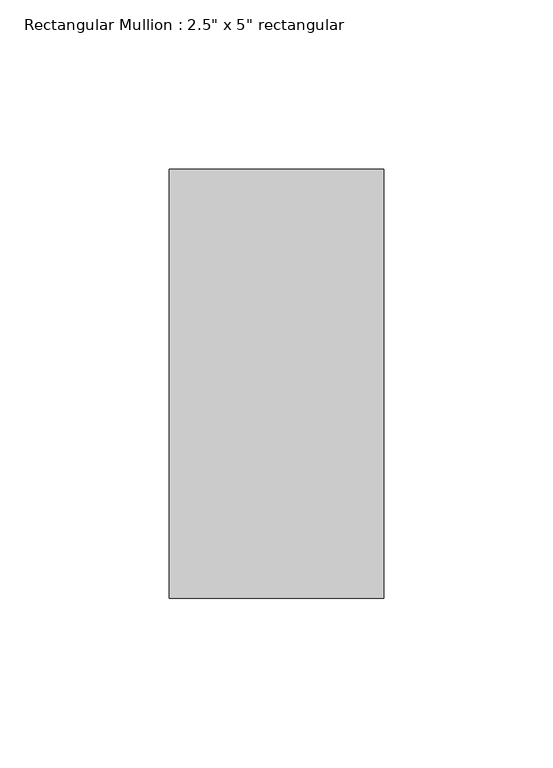
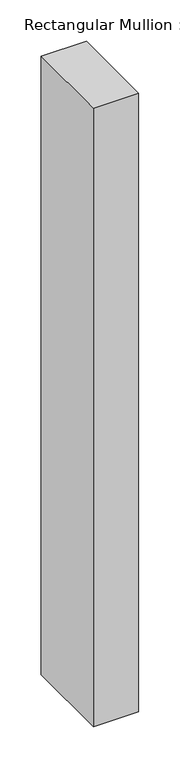
"""IFC4 building model written with IfcOpenShell, lengths in millimetres: member geometry."""

from ifc_helpers import new_model, si_unit, frame, origin, place, context, project, spatial, polyline, outline, extrude, source, transform, mapped, element, save


def member_6a93b315(model_context):
    return source(origin(), model_context, "Body", "SweptSolid", [
        extrude(outline(polyline([(0.0, 63.5), (0.0, -63.5), (-63.5, -63.5), (-63.5, 63.5), (0.0, 63.5)])), frame((0.0, 0.0, -916.1761324), z_axis=(0.0, 0.0, 1.0), x_axis=(1.0, 0.0, 0.0)), (0.0, 0.0, 1.0), 916.1761324),
    ])


if __name__ == "__main__":
    model = new_model("IFC4")
    model_context = context("Model", 3, world=origin())
    ifc_project = project(units=[si_unit("LENGTHUNIT", "METRE", prefix="MILLI")], contexts=[model_context])
    site = spatial("IfcSite", under=ifc_project)
    building = spatial("IfcBuilding", under=site)
    placement = place(None, origin())
    member_shape = member_6a93b315(model_context)
    element("IfcMember", 1, ObjectType="Rectangular Mullion : 2.5\" x 5\" rectangular", at=placement, inside=building, context=model_context, shape_type="MappedRepresentation", body=[
        mapped(member_shape, transform((0.0, 0.0, 0.0), x_axis=(1.0, 0.0, 0.0), y_axis=(0.0, 1.0, 0.0), z_axis=(0.0, 0.0, 1.0))),
    ])
    save(model, "model.ifc")

# Revit data of these elements
# Type "Rectangular Mullion : 2.5\" x 5\" rectangular"
#   built-in parameter 1007304 = 0.416667 (stored number, unit not read)
#   built-in parameter 1007301 = 0.104167 (stored number, unit not read)
#   built-in parameter 1007300 = 0.104167 (stored number, unit not read)
# Element 1 (IfcMember, "Rectangular Mullion : 2.5\" x 5\" rectangular")
#   Materials on its faces: "Aluminum"
# Materials
#   "Aluminum": class "Metal", colour RGB 247 247 247, transparency 0, Description = "Aluminum 6061", Cost = 0
